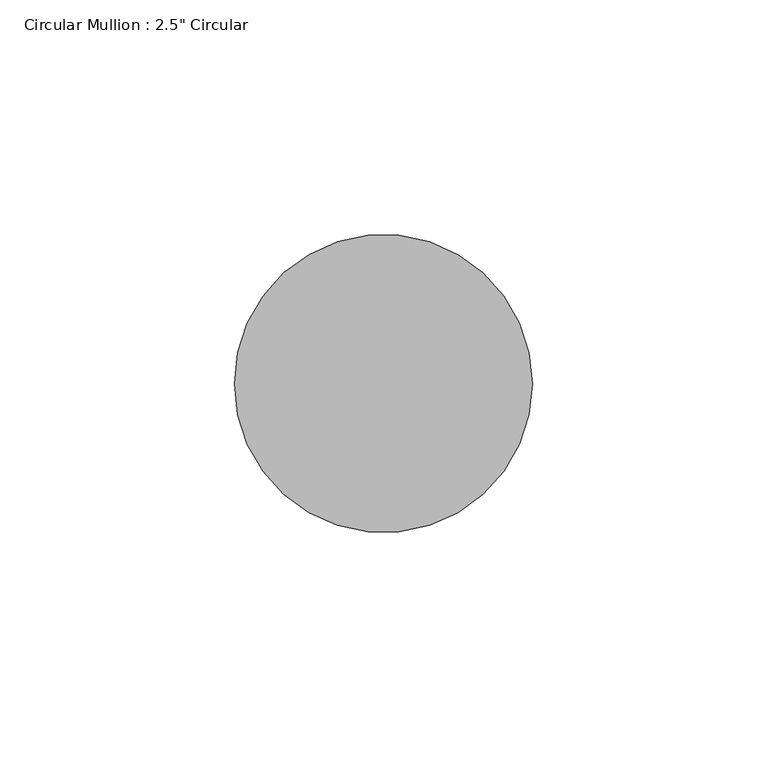
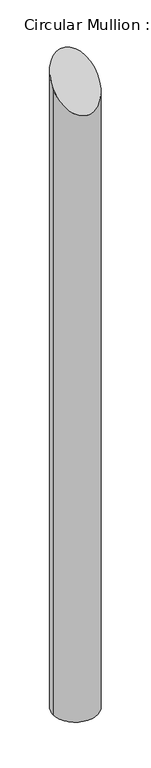
"""IFC4 building model written with IfcOpenShell, lengths in millimetres: member geometry."""

from ifc_helpers import new_model, si_unit, frame, origin, place, context, project, spatial, circle_curve, ellipse_curve, source, transform, mapped, element, save
from ifc_brep_helpers import plane_surface, cylinder_surface, advanced_brep


def member_72629bea(model_context):
    return source(origin(), model_context, "Body", "AdvancedBrep", [
        advanced_brep(
        [(0.0, 0.0, -944.5625), (-63.5, 0.0, -944.5625), (-63.5, 0.0, 0.0), (0.0, 0.0, 0.0)],
        [
            (0, 1, circle_curve(frame((-31.75, 0.0, -944.5625), z_axis=(0.0, 0.0, -1.0), x_axis=(1.0, 0.0, 0.0)), 31.75)),
            (1, 0, circle_curve(frame((-31.75, 0.0, -944.5625), z_axis=(0.0, 0.0, -1.0), x_axis=(1.0, 0.0, 0.0)), 31.75)),
            (2, 3, ellipse_curve(frame((-31.75, 0.0, 0.0), z_axis=(0.0, 0.707106781186547, -0.7071067811865481), x_axis=(0.0, 0.7071067811865481, 0.7071067811865468)), 44.9012806, 31.75)),
            (3, 0),
            (1, 2),
            (3, 2, ellipse_curve(frame((-31.75, 0.0, 0.0), z_axis=(0.0, 0.707106781186547, -0.7071067811865481), x_axis=(0.0, 0.7071067811865481, 0.7071067811865468)), 44.9012806, 31.75)),
        ],
        [
            plane_surface(frame((0.0, -63.5, -944.5625), z_axis=(0.0, 0.0, -1.0), x_axis=(-1.0, 0.0, 0.0))),
            cylinder_surface(frame((-31.75, 0.0, 0.0), z_axis=(0.0, 0.0, 1.0), x_axis=(1.0, 0.0, 0.0)), 31.75),
            plane_surface(frame((304.8, 0.0, 0.0), z_axis=(0.0, -0.707106781186547, 0.7071067811865481), x_axis=(0.0, -0.7071067811865481, -0.707106781186547))),
        ],
        [
            (0, [[1, 2]]),
            (1, [[3, 4, -2, 5]]),
            (1, [[6, -5, -1, -4]]),
            (2, [[-3, -6]]),
        ],
    ),
    ])


if __name__ == "__main__":
    model = new_model("IFC4")
    model_context = context("Model", 3, world=origin())
    ifc_project = project(units=[si_unit("LENGTHUNIT", "METRE", prefix="MILLI")], contexts=[model_context])
    site = spatial("IfcSite", under=ifc_project)
    building = spatial("IfcBuilding", under=site)
    placement = place(None, origin())
    member_shape = member_72629bea(model_context)
    element("IfcMember", 1, ObjectType="Circular Mullion : 2.5\" Circular", at=placement, inside=building, context=model_context, shape_type="MappedRepresentation", body=[
        mapped(member_shape, transform((0.0, 0.0, 0.0), x_axis=(1.0, 0.0, 0.0), y_axis=(0.0, 1.0, 0.0), z_axis=(0.0, 0.0, 1.0))),
    ])
    save(model, "model.ifc")

# Revit data of these elements
# Type "Circular Mullion : 2.5\" Circular"
#   built-in parameter 1007350 = 0.104167 (stored number, unit not read)
# Element 1 (IfcMember, "Circular Mullion : 2.5\" Circular")
#   Materials on its faces: "Aluminum"
# Materials
#   "Aluminum": class "Metal", colour RGB 247 247 247, transparency 0, Description = "Aluminum 6061", Cost = 0
